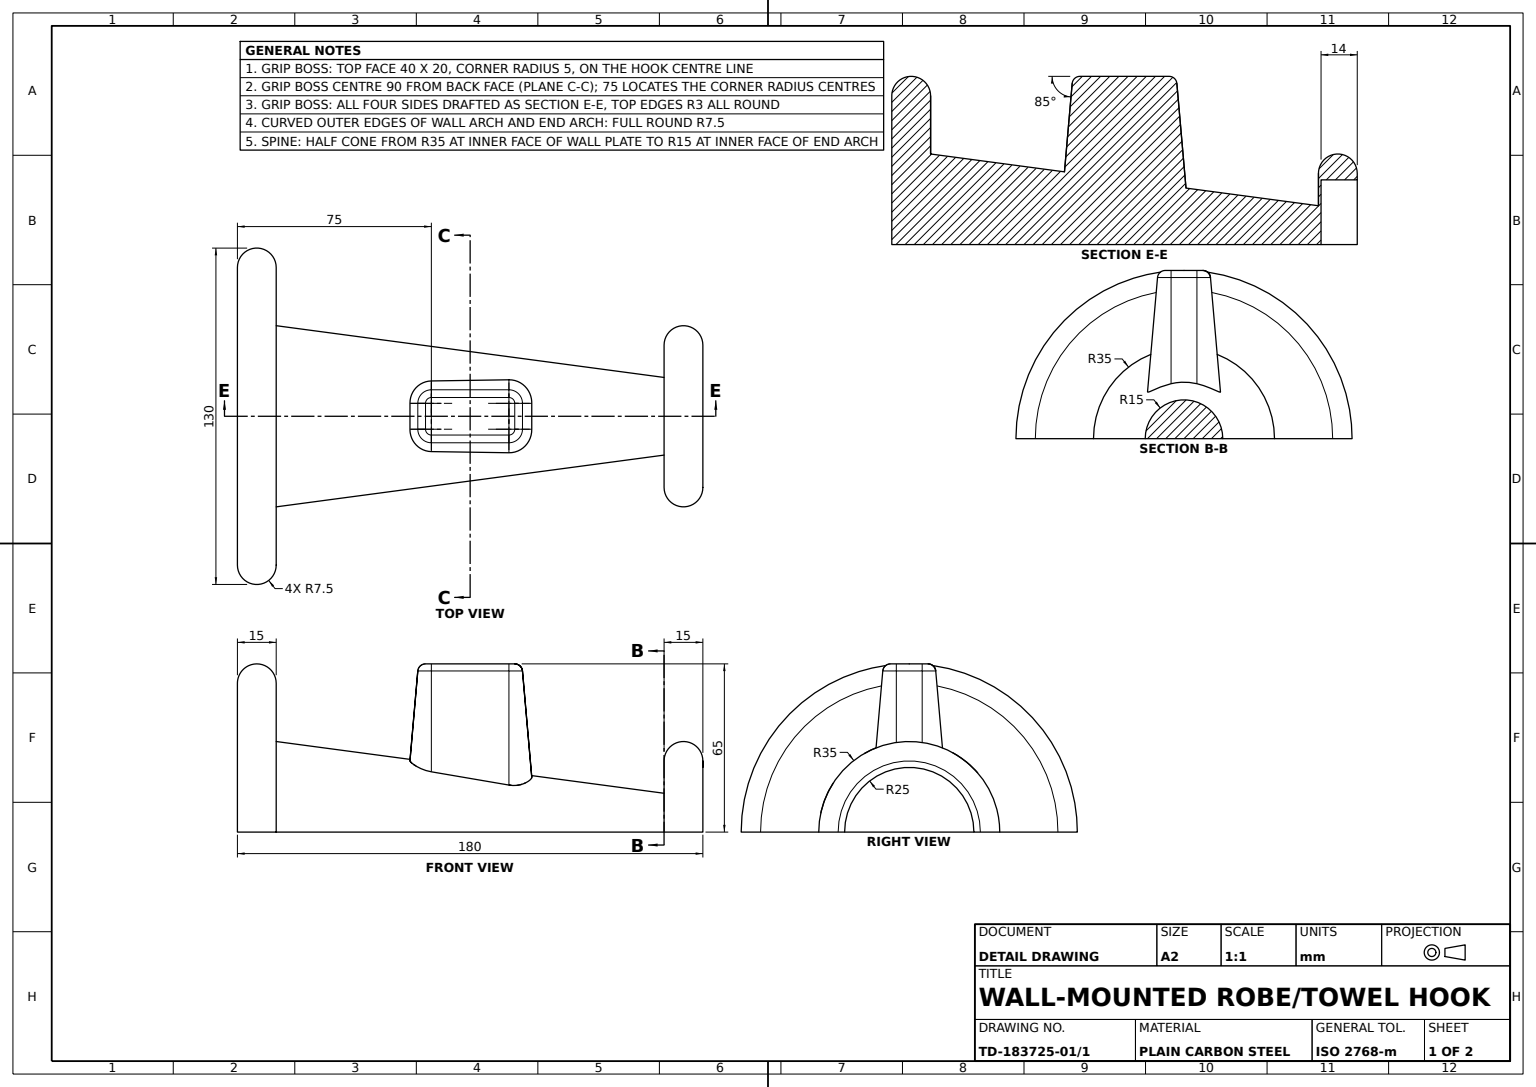
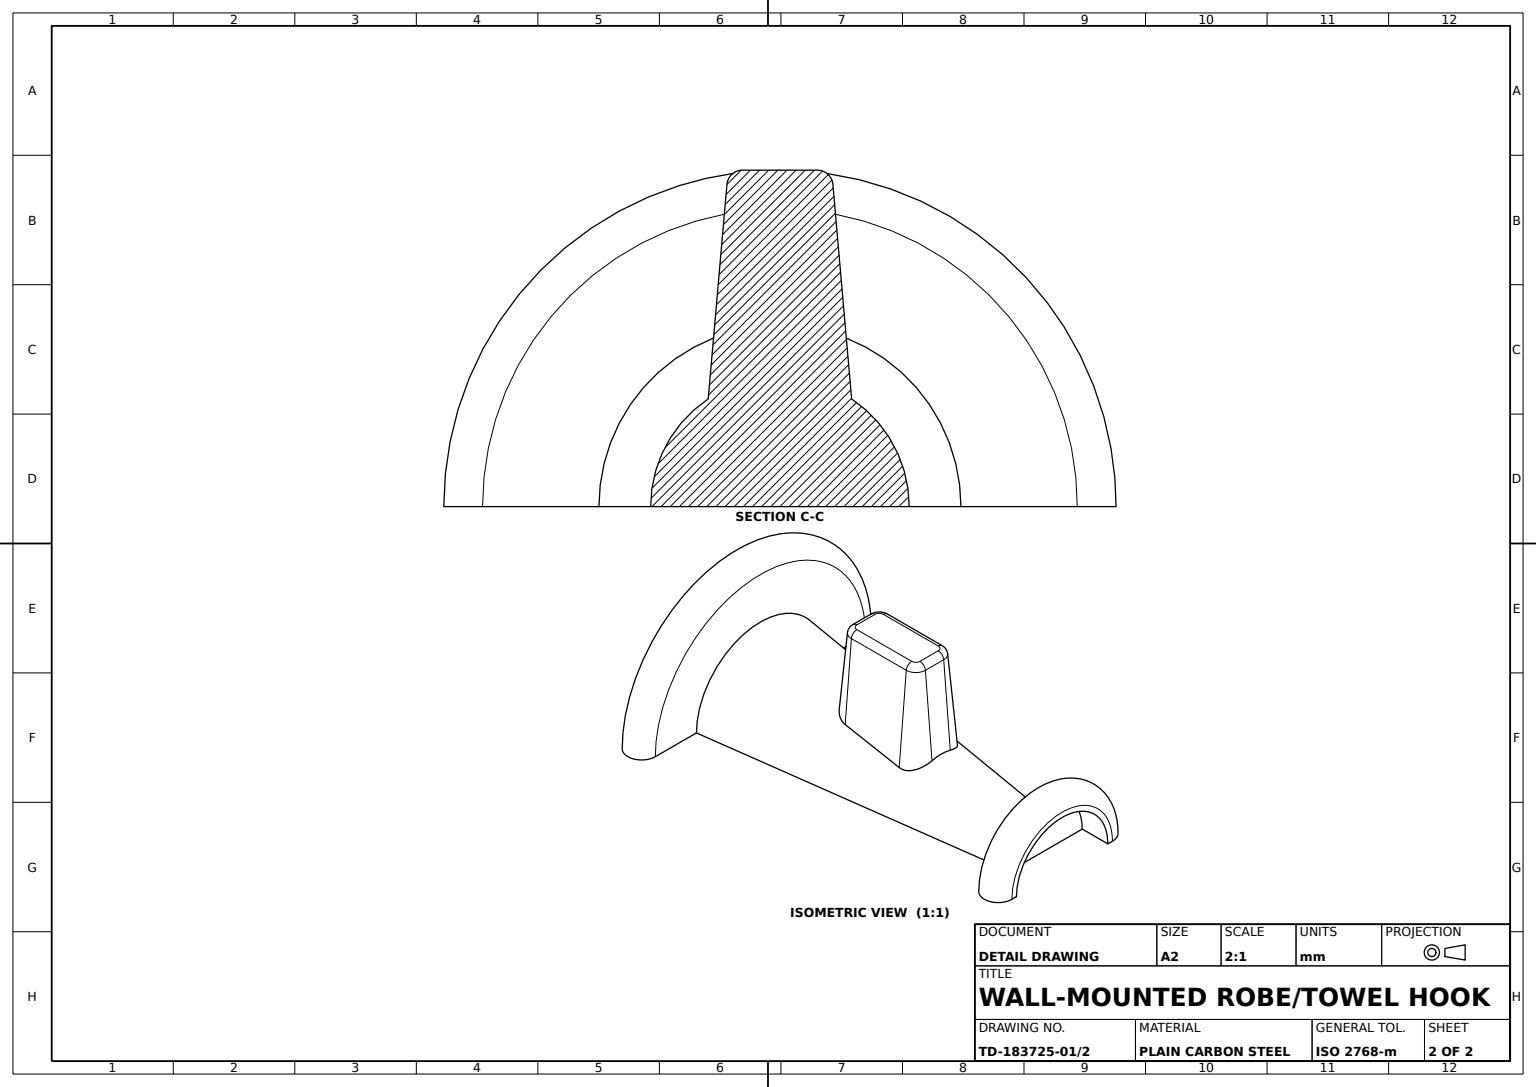
from build123d import *

# Parameters (mm, degrees)
HALF_SPLIT_CUT_DEPTH         = 94
HALF_SPLIT_CUT_DEPTH_BACK    = 80
HALF_SPLIT_CUT_SKETCH_W      = 233.621052632
HALF_SPLIT_CUT_SKETCH_H      = 71.905263158
GRIP_BOSS_DRAFTED_5DEG_DEPTH = 65
GRIP_BOSS_DRAFTED_5DEG_DRAFT = 5
GRIP_BOSS_FILLET_R3_R        = 3
HOOK_END_RECESS_SKETCH_50_R  = 25
HOOK_END_RECESS_50X14_DEPTH  = 14


with BuildPart() as part:
    # Hook Body Profile → Hook Body Revolve (revolve)
    with BuildSketch(Plane.XY, mode=Mode.PRIVATE) as hook_body_revolve_sk:
        with BuildLine():
            Line((-90, 0), (-75, 0))
            Line((-75, 0), (-75, 35))
            Line((-75, 35), (-75, 57.5))
            ThreePointArc((-75, 57.5), (-82.5, 65), (-90, 57.5))
            Line((-90, 57.5), (-90, 0))
        make_face()
        Polygon((-75, 0), (0, 0), (75, 0), (75, 15), (-75, 35), align=None)
        with BuildLine():
            Line((75, 15), (75, 0))
            Line((75, 0), (90, 0))
            Line((90, 0), (90, 27.5))
            ThreePointArc((90, 27.5), (82.5, 35), (75, 27.5))
            Line((75, 27.5), (75, 15))
        make_face()
    revolve(hook_body_revolve_sk.sketch.rotate(Axis((0, 0, 0), (1, 0, 0)), 90), axis=Axis((0, 0, 0), (1, 0, 0)))

    # Half Split Cut Sketch → Half Split Cut (cut, two sides: drawn at the far end of the back side and taken through both)
    with BuildSketch(Plane.XY.offset(-HALF_SPLIT_CUT_DEPTH_BACK)):
        with Locations((-1.705263158, -35.952631579)):
            Rectangle(HALF_SPLIT_CUT_SKETCH_W, HALF_SPLIT_CUT_SKETCH_H)
    extrude(amount=HALF_SPLIT_CUT_DEPTH + HALF_SPLIT_CUT_DEPTH_BACK, mode=Mode.SUBTRACT)


with BuildPart() as grip_boss_drafted_5deg_tool:
    # Grip Boss Sketch 40x20 → Grip Boss Drafted 5deg (with draft: the straight prism first)
    with BuildSketch(Plane(origin=(0, 65, 0), x_dir=(1, 0, 0), z_dir=(0, 1, 0))):
        with BuildLine():
            ThreePointArc((-15, 10), (-18.535533906, 8.535533906), (-20, 5))
            Line((-20, 5), (-20, -5))
            ThreePointArc((-20, -5), (-18.535533906, -8.535533906), (-15, -10))
            Line((-15, -10), (15, -10))
            ThreePointArc((15, -10), (18.535533906, -8.535533906), (20, -5))
            Line((20, -5), (20, 5))
            ThreePointArc((20, 5), (18.535533906, 8.535533906), (15, 10))
            Line((15, 10), (-15, 10))
        make_face()
    extrude(amount=-GRIP_BOSS_DRAFTED_5DEG_DEPTH)
    # Grip Boss Drafted 5deg: the draft: its side faces are tilted about the plane it starts from
    grip_boss_drafted_5deg_sides = [grip_boss_drafted_5deg_tool.faces().sort_by_distance(p)[0] for p in [
        (-18.535533906, 32.5, -8.535533906),
        (-20, 32.5, 0),
        (-18.535533906, 32.5, 8.535533906),
        (0, 32.5, 10),
        (18.535533906, 32.5, 8.535533906),
        (20, 32.5, 0),
        (18.535533906, 32.5, -8.535533906),
        (0, 32.5, -10),
    ]]
    draft(grip_boss_drafted_5deg_sides, Plane(origin=(0, 65, 0), x_dir=(1, 0, 0), z_dir=(0, 1, 0)), GRIP_BOSS_DRAFTED_5DEG_DRAFT)


with BuildPart() as part_1:
    add(part.part)

    # Grip Boss Drafted 5deg: add grip_boss_drafted_5deg_tool
    add(grip_boss_drafted_5deg_tool.part)

    # Grip Boss Fillet R3
    grip_boss_fillet_r3_edges = [part_1.edges().sort_by_distance(p)[0] for p in [
        (18.535533906, 65, -8.535533906),
        (0, 65, -10),
        (-18.535533906, 65, -8.535533906),
        (-20, 65, 0),
        (-18.535533906, 65, 8.535533906),
        (0, 65, 10),
        (18.535533906, 65, 8.535533906),
        (20, 65, 0),
    ]]
    fillet(grip_boss_fillet_r3_edges, radius=GRIP_BOSS_FILLET_R3_R)

    # Hook End Recess Sketch Ø50 → Hook End Recess Ø50x14 (cut)
    with BuildSketch(Plane(origin=(90, 0, 0), x_dir=(0, 0, -1), z_dir=(1, 0, 0))):
        Circle(HOOK_END_RECESS_SKETCH_50_R)
    extrude(amount=-HOOK_END_RECESS_50X14_DEPTH, mode=Mode.SUBTRACT)


solid = part_1.part
